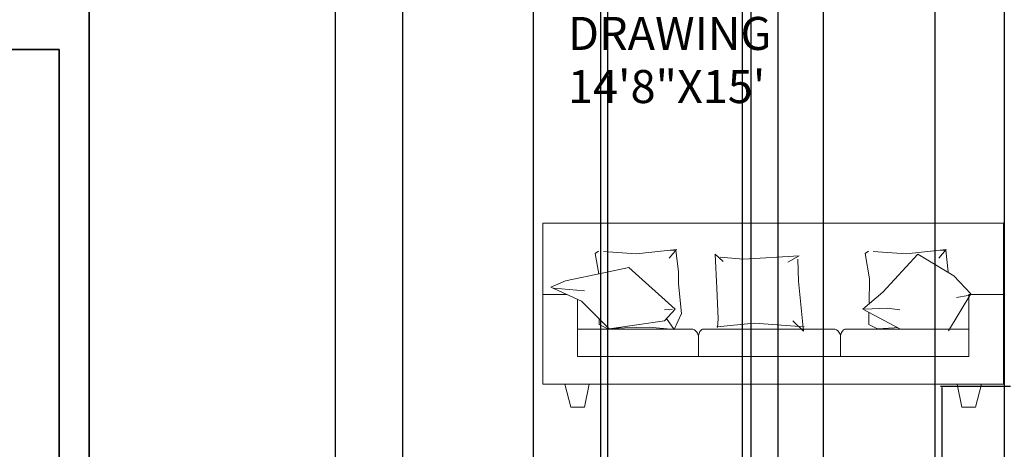
# Model space of a CAD drawing. Units: inches. Extents: x -26 to 385, y 12 to 697.
# Tile 9 of 13: x 136 to 285, y 215 to 280. Entities that reach past the tile are written whole.
import ezdxf

# ---------------------------------------------------------------- set-up
doc = ezdxf.new("R2010")
doc.units = ezdxf.units.IN
doc.header["$MEASUREMENT"] = 0
for name, color, linetype, lineweight in [('A-ANNO-DIMS', 4, 'Continuous', 18), ('A-AREA-IDEN', 4, 'Continuous', 18), ('A-WALL', 40, 'Continuous', 35), ('Furniture', 210, 'Continuous', 15)]:
    doc.layers.add(name, color=color, linetype=linetype, lineweight=lineweight)
doc.styles.get("Standard").update_dxf_attribs({"font": 'italic8.shx'})
doc.dimstyles.get("Standard").update_dxf_attribs({"dimtxt": 8, "dimasz": 0.18, "dimexe": 0.18, "dimexo": 0.0625, "dimgap": 0.09, "dimtad": 0, "dimtih": 1, "dimtoh": 1, "dimdec": 4, "dimzin": 0, "dimdsep": 46, "dimlunit": 3, "dimtxsty": 'Standard', "dimcen": 0.09, "dimclrd": 2, "dimclre": 3, "dimclrt": 6, "dimadec": 0, "dimazin": 0, "dimtfac": 1, "dimtdec": 4, "dimtofl": 0, "dimtmove": 0, "dimatfit": 3, "dimfxl": 1, "dimtolj": 1, "dimtzin": 0, "dimarcsym": 0})

# ---------------------------------------------------------------- blocks, each defined once
blk = doc.blocks.new('SOFA-THREE-SEAT')
for p, q in [((-5.22, 20.2), (64.44, 20.2)), ((-5.22, 20.2), (-5.22, -4.18)), ((64.44, 20.2), (64.44, -4.18)), ((2.7, 15.63), (3.2, 15.97)), ((3.23, 12.52), (2.7, 15.63)), ((3.92, 15.91), (8.89, 15.54)), ((8.89, 15.54), (14.99, 16.19)), ((14.99, 16.19), (13.87, 14.88)), ((14.06, 16.09), (14.9, 16.1)), ((14.9, 16.1), (15.27, 12.82)), ((21.11, 10.37), (20.83, 15.51)), ((20.83, 15.51), (22.04, 14.39)), ((21.58, 15.04), (25.13, 14.76)), ((25.13, 14.76), (33.53, 15.23)), ((33.53, 15.23), (31.85, 14.29)), ((43.52, 15.63), (44.02, 15.97)), ((44.18, 11.79), (43.52, 15.63)), ((44.74, 15.91), (49.71, 15.54)), ((46.2, 9.78), (51.51, 15.49)), ((49.71, 15.54), (55.81, 16.19)), ((51.51, 15.49), (56.95, 12.22)), ((55.81, 16.19), (54.69, 14.88)), ((54.88, 16.09), (55.72, 16.1)), ((55.72, 16.1), (56.09, 12.82)), ((7.78, 13.51), (3.97, 12.67)), ((14.76, 7.19), (7.78, 13.51)), ((33.35, 14.76), (33.44, 11.4)), ((3.97, 12.67), (-1.8, 11.46)), ((15.27, 12.82), (15.27, 11.04)), ((56.09, 12.82), (56.09, 12.74)), ((56.95, 12.22), (59.54, 9.5)), ((-1.8, 11.46), (-4.04, 10.53)), ((-4.04, 10.53), (0.62, 8.39)), ((15.27, 11.04), (15.74, 6.54)), ((33.44, 11.4), (34.19, 3.84)), ((44.12, 7.99), (44.18, 11.79)), ((-5.22, 9.4), (-1.58, 9.4)), ((-3.57, 10.35), (1.08, 9.97)), ((21.3, 5.71), (21.11, 10.37)), ((43.2, 7.19), (46.2, 9.78)), ((59.54, 9.5), (56.14, 3.93)), ((59.13, 9.23), (57.36, 8.96)), ((59.21, 9.4), (59.21, 0)), ((59.21, 9.4), (64.44, 9.4)), ((0, 8.68), (0, 0)), ((0.62, 8.39), (4.8, 4.21)), ((14.39, 7.19), (13.18, 7.09)), ((13.18, 5.42), (14.76, 7.19)), ((15.74, 6.54), (14.62, 4.1)), ((48.79, 4.2), (43.2, 7.19)), ((43.48, 7.19), (46.88, 7.33)), ((44.08, 4.85), (44.11, 6.71)), ((46.88, 7.33), (48.79, 7.06)), ((3.26, 4.85), (3.27, 5.74)), ((4.57, 4.19), (3.26, 4.85)), ((4.8, 4.21), (13.18, 5.42)), ((10.86, 4.47), (7.11, 4.38)), ((14.62, 4.1), (10.86, 4.47)), ((14.62, 4.1), (13.47, 5.75)), ((21.11, 4.5), (26.81, 5.06)), ((21.2, 4.4), (21.3, 5.71)), ((26.81, 5.06), (34.28, 4.5)), ((34.19, 3.84), (32.6, 5.43)), ((45.4, 4.19), (44.08, 4.85)), ((0, 4.18), (17.44, 4.18)), ((7.11, 4.38), (4.57, 4.19)), ((18.3, 3.23), (18.3, 0)), ((18.93, 4.18), (38.96, 4.18)), ((39.82, 3.23), (39.82, 0)), ((40.44, 4.18), (59.21, 4.18)), ((47.93, 4.38), (45.4, 4.19)), ((48.43, 4.39), (47.93, 4.38)), ((0, 0), (59.21, 0)), ((-5.22, -4.18), (64.44, -4.18)), ((-1.91, -4.18), (-1.01, -7.66)), ((1.75, -4.18), (1.07, -7.66)), ((57.47, -4.18), (58.14, -7.66)), ((61.12, -4.18), (60.22, -7.66)), ((-1.01, -7.66), (1.07, -7.66)), ((58.14, -7.66), (60.22, -7.66))]:
    blk.add_line(p, q)
for points, knots in [([(17.44, 4.18), (17.62, 4.1), (18, 3.87), (18.2, 3.46), (18.3, 3.23)], [15.247039, 15.247039, 15.247039, 15.247039, 32.166322, 53.547435, 53.547435, 53.547435, 53.547435]), ([(18.3, 3.22), (18.36, 3.42), (18.48, 3.8), (18.78, 4.06), (18.93, 4.18)], [5.353258, 5.353258, 5.353258, 5.353258, 23.098733, 39.167876, 39.167876, 39.167876, 39.167876]), ([(38.96, 4.18), (39.14, 4.1), (39.51, 3.87), (39.71, 3.46), (39.82, 3.23)], [15.247039, 15.247039, 15.247039, 15.247039, 32.166322, 53.547435, 53.547435, 53.547435, 53.547435]), ([(39.82, 3.22), (39.87, 3.42), (39.99, 3.8), (40.29, 4.06), (40.44, 4.18)], [5.353258, 5.353258, 5.353258, 5.353258, 23.098733, 39.167876, 39.167876, 39.167876, 39.167876])]:
    blk.add_open_spline(points, degree=3, knots=knots)
blk = doc.blocks.new('*D11')
at = {"layer": 'A-ANNO-DIMS', "color": 3, "lineweight": -2, "transparency": 16777216}
for p, q in [((285.56, 224.4), (274.99, 224.4)), ((285.56, 154.74), (274.99, 154.74))]:
    blk.add_line(p, q, dxfattribs=at)
at = {"layer": 'A-ANNO-DIMS', "color": 2, "lineweight": -2, "transparency": 16777216}
for p, q in [((275.17, 224.22), (275.17, 195.75)), ((275.17, 154.92), (275.17, 183.38))]:
    blk.add_line(p, q, dxfattribs=at)
at = {"layer": 'A-ANNO-DIMS', "color": 2, "transparency": 16777216}
for points in [[(275.14, 224.22), (275.2, 224.22), (275.17, 224.4)], [(275.14, 154.92), (275.2, 154.92), (275.17, 154.74)]]:
    blk.add_solid(points, dxfattribs=at)
at = {"layer": 'Defpoints', "color": 0, "transparency": 16777216}
for p in [(285.62, 224.4), (275.17, 154.74), (285.62, 154.74)]:
    blk.add_point(p, dxfattribs=at)
at = {"layer": 'A-ANNO-DIMS', "color": 6, "transparency": 16777216, "insert": (275.17, 189.57), "char_height": 8, "attachment_point": 5}
blk.add_mtext('\\A1;SOFA 5\'-9 1/2" TYP.', dxfattribs=at)
blk = doc.blocks.new('*D25')
at = {"layer": 'A-ANNO-DIMS', "color": 3, "lineweight": -2, "transparency": 16777216}
for p, q in [((284.629322, 368.316588), (284.629322, 23.949088)), ((320.629322, 368.316588), (320.629322, 23.949088))]:
    blk.add_line(p, q, dxfattribs=at)
at = {"layer": 'A-ANNO-DIMS', "color": 2, "lineweight": -2, "transparency": 16777216}
for p, q in [((284.449322, 24.129088), (284.269322, 24.129088)), ((320.809322, 24.129088), (320.989322, 24.129088))]:
    blk.add_line(p, q, dxfattribs=at)
at = {"layer": 'A-ANNO-DIMS', "color": 2, "transparency": 16777216}
for points in [[(284.449322, 24.159088), (284.449322, 24.099088), (284.629322, 24.129088)], [(320.809322, 24.159088), (320.809322, 24.099088), (320.629322, 24.129088)]]:
    blk.add_solid(points, dxfattribs=at)
at = {"layer": 'Defpoints', "color": 0, "transparency": 16777216}
for p in [(284.629322, 368.379088), (320.629322, 368.379088), (320.629322, 24.129088)]:
    blk.add_point(p, dxfattribs=at)
at = {"layer": 'A-ANNO-DIMS', "color": 6, "transparency": 16777216, "insert": (302.629322, 24.129088), "char_height": 8, "attachment_point": 5}
blk.add_mtext('\\A1;3\'-0"', dxfattribs=at)
blk = doc.blocks.new('*D33')
at = {"layer": 'A-ANNO-DIMS', "color": 3, "lineweight": -2, "transparency": 16777216}
for p, q in [((58.47, 279.82), (58.47, 23.95)), ((97.85, 279.82), (97.85, 23.95))]:
    blk.add_line(p, q, dxfattribs=at)
at = {"layer": 'A-ANNO-DIMS', "color": 2, "lineweight": -2, "transparency": 16777216}
for p, q in [((58.65, 24.13), (97.67, 24.13)), ((97.85, 24.13), (98.03, 24.13))]:
    blk.add_line(p, q, dxfattribs=at)
at = {"layer": 'A-ANNO-DIMS', "color": 2, "transparency": 16777216}
for points in [[(58.65, 24.16), (58.65, 24.1), (58.47, 24.13)], [(97.67, 24.16), (97.67, 24.1), (97.85, 24.13)]]:
    blk.add_solid(points, dxfattribs=at)
at = {"layer": 'Defpoints', "color": 0, "transparency": 16777216}
for p in [(58.47, 279.88), (97.85, 279.88), (97.85, 24.13)]:
    blk.add_point(p, dxfattribs=at)
at = {"layer": 'A-ANNO-DIMS', "color": 6, "transparency": 16777216, "insert": (131.26, 24.13), "char_height": 8, "attachment_point": 5}
blk.add_mtext('\\A1;3\'-3 1/2"', dxfattribs=at)
blk = doc.blocks.new('*D35')
at = {"layer": 'A-ANNO-DIMS', "color": 3, "lineweight": -2, "transparency": 16777216}
for p, q in [((193.6, 147.94), (193.6, 684.81)), ((244.99, 147.94), (244.99, 684.81))]:
    blk.add_line(p, q, dxfattribs=at)
at = {"layer": 'A-ANNO-DIMS', "color": 2, "lineweight": -2, "transparency": 16777216}
for p, q in [((193.78, 684.63), (244.81, 684.63)), ((244.99, 684.63), (245.17, 684.63))]:
    blk.add_line(p, q, dxfattribs=at)
at = {"layer": 'A-ANNO-DIMS', "color": 2, "transparency": 16777216}
for points in [[(193.78, 684.66), (193.78, 684.6), (193.6, 684.63)], [(244.81, 684.66), (244.81, 684.6), (244.99, 684.63)]]:
    blk.add_solid(points, dxfattribs=at)
at = {"layer": 'Defpoints', "color": 0, "transparency": 16777216}
for p in [(244.99, 684.63), (193.6, 147.88), (244.99, 147.88)]:
    blk.add_point(p, dxfattribs=at)
at = {"layer": 'A-ANNO-DIMS', "color": 6, "transparency": 16777216, "insert": (278.4, 684.63), "char_height": 8, "attachment_point": 5}
blk.add_mtext('\\A1;4\'-3 1/2"', dxfattribs=at)
blk = doc.blocks.new('*D36')
at = {"layer": 'A-ANNO-DIMS', "color": 3, "lineweight": -2, "transparency": 16777216}
for p, q in [((146.13, 147.94), (146.13, 684.81)), ((193.6, 147.94), (193.6, 684.81))]:
    blk.add_line(p, q, dxfattribs=at)
at = {"layer": 'A-ANNO-DIMS', "color": 2, "lineweight": -2, "transparency": 16777216}
for p, q in [((146.31, 684.63), (193.42, 684.63)), ((193.6, 684.63), (193.78, 684.63))]:
    blk.add_line(p, q, dxfattribs=at)
at = {"layer": 'A-ANNO-DIMS', "color": 2, "transparency": 16777216}
for points in [[(146.31, 684.66), (146.31, 684.6), (146.13, 684.63)], [(193.42, 684.66), (193.42, 684.6), (193.6, 684.63)]]:
    blk.add_solid(points, dxfattribs=at)
at = {"layer": 'Defpoints', "color": 0, "transparency": 16777216}
for p in [(193.6, 684.63), (146.13, 147.88), (193.6, 147.88)]:
    blk.add_point(p, dxfattribs=at)
at = {"layer": 'A-ANNO-DIMS', "color": 6, "transparency": 16777216, "insert": (228.34, 684.63), "char_height": 8, "attachment_point": 5}
blk.add_mtext('\\A1;3\'-11 1/2"', dxfattribs=at)
blk = doc.blocks.new('*D37')
at = {"layer": 'A-ANNO-DIMS', "color": 3, "lineweight": -2, "transparency": 16777216}
for p, q in [((223.55, 597.32), (223.55, 23.95)), ((257.22, 597.32), (257.22, 23.95))]:
    blk.add_line(p, q, dxfattribs=at)
at = {"layer": 'A-ANNO-DIMS', "color": 2, "lineweight": -2, "transparency": 16777216}
for p, q in [((223.73, 24.13), (257.04, 24.13)), ((257.22, 24.13), (257.4, 24.13))]:
    blk.add_line(p, q, dxfattribs=at)
at = {"layer": 'A-ANNO-DIMS', "color": 2, "transparency": 16777216}
for points in [[(223.73, 24.16), (223.73, 24.1), (223.55, 24.13)], [(257.04, 24.16), (257.04, 24.1), (257.22, 24.13)]]:
    blk.add_solid(points, dxfattribs=at)
at = {"layer": 'Defpoints', "color": 0, "transparency": 16777216}
for p in [(223.55, 597.38), (257.22, 597.38), (257.22, 24.13)]:
    blk.add_point(p, dxfattribs=at)
at = {"layer": 'A-ANNO-DIMS', "color": 6, "transparency": 16777216, "insert": (290.63, 24.13), "char_height": 8, "attachment_point": 5}
blk.add_mtext('\\A1;2\'-9 1/2"', dxfattribs=at)
blk = doc.blocks.new('*D39')
at = {"layer": 'A-ANNO-DIMS', "color": 3, "lineweight": -2, "transparency": 16777216}
for p, q in [((183.36, 597.32), (183.36, 23.95)), ((213.36, 597.32), (213.36, 23.95))]:
    blk.add_line(p, q, dxfattribs=at)
at = {"layer": 'A-ANNO-DIMS', "color": 2, "lineweight": -2, "transparency": 16777216}
for p, q in [((183.54, 24.13), (213.18, 24.13)), ((213.36, 24.13), (213.54, 24.13))]:
    blk.add_line(p, q, dxfattribs=at)
at = {"layer": 'A-ANNO-DIMS', "color": 2, "transparency": 16777216}
for points in [[(183.54, 24.16), (183.54, 24.1), (183.36, 24.13)], [(213.18, 24.16), (213.18, 24.1), (213.36, 24.13)]]:
    blk.add_solid(points, dxfattribs=at)
at = {"layer": 'Defpoints', "color": 0, "transparency": 16777216}
for p in [(183.36, 597.38), (213.36, 597.38), (213.36, 24.13)]:
    blk.add_point(p, dxfattribs=at)
at = {"layer": 'A-ANNO-DIMS', "color": 6, "transparency": 16777216, "insert": (231.53, 24.13), "char_height": 8, "attachment_point": 5}
blk.add_mtext('\\A1;2\'-6"', dxfattribs=at)
blk = doc.blocks.new('*D42')
at = {"layer": 'A-ANNO-DIMS', "color": 3, "lineweight": -2, "transparency": 16777216}
for p, q in [((250.37, 518.99), (250.37, 23.95)), ((274.13, 518.99), (274.13, 23.95))]:
    blk.add_line(p, q, dxfattribs=at)
at = {"layer": 'A-ANNO-DIMS', "color": 2, "lineweight": -2, "transparency": 16777216}
for p, q in [((250.55, 24.13), (273.95, 24.13)), ((274.13, 24.13), (274.31, 24.13))]:
    blk.add_line(p, q, dxfattribs=at)
at = {"layer": 'A-ANNO-DIMS', "color": 2, "transparency": 16777216}
for points in [[(250.55, 24.16), (250.55, 24.1), (250.37, 24.13)], [(273.95, 24.16), (273.95, 24.1), (274.13, 24.13)]]:
    blk.add_solid(points, dxfattribs=at)
at = {"layer": 'Defpoints', "color": 0, "transparency": 16777216}
for p in [(250.37, 519.05), (274.13, 519.05), (274.13, 24.13)]:
    blk.add_point(p, dxfattribs=at)
at = {"layer": 'A-ANNO-DIMS', "color": 6, "transparency": 16777216, "insert": (292.3, 24.13), "char_height": 8, "attachment_point": 5}
blk.add_mtext('\\A1;2\'-0"', dxfattribs=at)
blk = doc.blocks.new('*D46')
at = {"layer": 'A-ANNO-DIMS', "color": 3, "lineweight": -2, "transparency": 16777216}
for p, q in [((224.59, 477.32), (224.59, 23.95)), ((284.63, 477.32), (284.63, 23.95))]:
    blk.add_line(p, q, dxfattribs=at)
at = {"layer": 'A-ANNO-DIMS', "color": 2, "lineweight": -2, "transparency": 16777216}
for p, q in [((224.77, 24.13), (236.62, 24.13)), ((284.45, 24.13), (272.61, 24.13))]:
    blk.add_line(p, q, dxfattribs=at)
at = {"layer": 'A-ANNO-DIMS', "color": 2, "transparency": 16777216}
for points in [[(224.77, 24.16), (224.77, 24.1), (224.59, 24.13)], [(284.45, 24.16), (284.45, 24.1), (284.63, 24.13)]]:
    blk.add_solid(points, dxfattribs=at)
at = {"layer": 'Defpoints', "color": 0, "transparency": 16777216}
for p in [(224.59, 477.38), (284.63, 477.38), (284.63, 24.13)]:
    blk.add_point(p, dxfattribs=at)
at = {"layer": 'A-ANNO-DIMS', "color": 6, "transparency": 16777216, "insert": (254.61, 24.13), "char_height": 8, "attachment_point": 5}
blk.add_mtext('\\A1;5\'-0"', dxfattribs=at)
blk = doc.blocks.new('*D50')
at = {"layer": 'A-ANNO-DIMS', "color": 3, "lineweight": -2, "transparency": 16777216}
for p, q in [((246.28, 401.87), (246.28, 23.95)), ((284.63, 398.32), (284.63, 23.95))]:
    blk.add_line(p, q, dxfattribs=at)
at = {"layer": 'A-ANNO-DIMS', "color": 2, "lineweight": -2, "transparency": 16777216}
for p, q in [((246.46, 24.13), (284.45, 24.13)), ((284.63, 24.13), (284.81, 24.13))]:
    blk.add_line(p, q, dxfattribs=at)
at = {"layer": 'A-ANNO-DIMS', "color": 2, "transparency": 16777216}
for points in [[(246.46, 24.16), (246.46, 24.1), (246.28, 24.13)], [(284.45, 24.16), (284.45, 24.1), (284.63, 24.13)]]:
    blk.add_solid(points, dxfattribs=at)
at = {"layer": 'Defpoints', "color": 0, "transparency": 16777216}
for p in [(246.28, 401.93), (284.63, 398.38), (284.63, 24.13)]:
    blk.add_point(p, dxfattribs=at)
at = {"layer": 'A-ANNO-DIMS', "color": 6, "transparency": 16777216, "insert": (318.04, 24.13), "char_height": 8, "attachment_point": 5}
blk.add_mtext('\\A1;3\'-2 1/2"', dxfattribs=at)

msp = doc.modelspace()

# ---------------------------------------------------------------- linework, layer by layer
at = {"layer": 'A-WALL'}
for p, q in [((146.12932, 332.37909), (146.12932, 194.90341)), ((141.62932, 275.37909), (29.62932, 275.37909)), ((141.62932, 275.37909), (141.62932, 194.90341))]:
    msp.add_line(p, q, dxfattribs=at)

# ---------------------------------------------------------------- block references
at = {"layer": 'Furniture'}
msp.add_blockref('SOFA-THREE-SEAT', (220.044, 228.904), dxfattribs=at)

# ---------------------------------------------------------------- texts
at = {"layer": 'A-AREA-IDEN'}
for s, p in [('DRAWING', (218.60931, 275.29915)), ('14\'8"X15\'', (218.60931, 267.26709))]:
    msp.add_text(s, height=5, dxfattribs=at).set_placement(p)

# ---------------------------------------------------------------- dimensions: what is measured, and where the dimension line sits
at = {"layer": 'A-ANNO-DIMS'}
for base, p1, p2, picture, middle in [((193.59818, 684.62909), (146.12932, 147.87909), (193.59818, 147.87909), '*D36', (228.34437, 684.62909)), ((244.98557, 684.62909), (193.59818, 147.87909), (244.98557, 147.87909), '*D35', (278.39843, 684.62909)), ((213.35855, 24.12909), (183.35855, 597.37909), (213.35855, 597.37909), '*D39', (231.53331, 24.12909)), ((257.21981, 24.12909), (223.54856, 597.37909), (257.21981, 597.37909), '*D37', (290.63267, 24.12909)), ((274.12932, 24.12909), (250.37102, 519.05498), (274.12932, 519.05498), '*D42', (292.30408, 24.12909)), ((284.62932, 24.12909), (224.59493, 477.37909), (284.62932, 477.37909), '*D46', (254.61213, 24.12909)), ((284.62932, 24.12909), (246.27828, 401.934), (284.62932, 398.37909), '*D50', (318.04218, 24.12909)), ((320.62932, 24.12909), (284.62932, 368.37909), (320.62932, 368.37909), '*D25', (302.62932, 24.12909)), ((97.84659, 24.12909), (58.46784, 279.87909), (97.84659, 279.87909), '*D33', (131.25945, 24.12909))]:
    dim = msp.add_linear_dim(base=base, p1=p1, p2=p2, dimstyle='Standard', override={"dimdec": 1, "dimlfac": 1, "dimrnd": 0, "dimzin": 1, "dimdsep": 46, "dimlunit": 4, "dimfrac": 2}, dxfattribs=at)
    dim.commit()
    dim.dimension.update_dxf_attribs({"geometry": picture, "text_midpoint": middle})
dim = msp.add_linear_dim(base=(275.17245, 154.73754), p1=(285.62207, 224.40165), p2=(285.62207, 154.73754), angle=270, text='SOFA <> TYP.', dimstyle='Standard', override={"dimdec": 1, "dimlfac": 1, "dimrnd": 0, "dimzin": 1, "dimdsep": 46, "dimlunit": 4, "dimfrac": 2}, dxfattribs=at)
dim.commit()
dim.dimension.update_dxf_attribs({"geometry": '*D11', "text_midpoint": (275.17245, 189.56959)})

doc.saveas('drawing.dxf')
